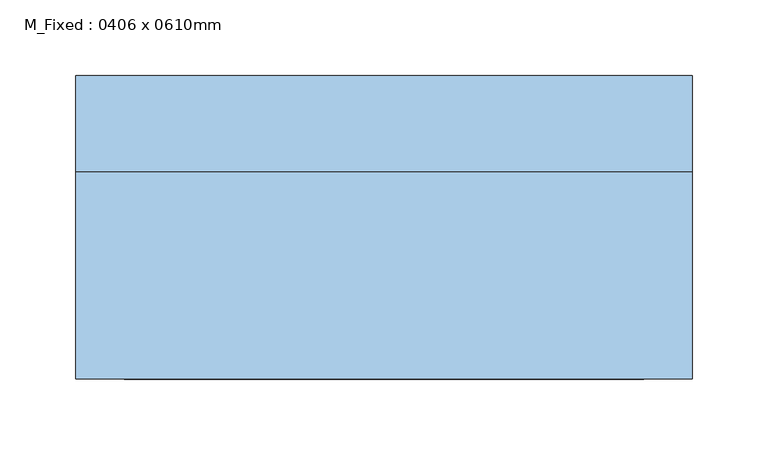
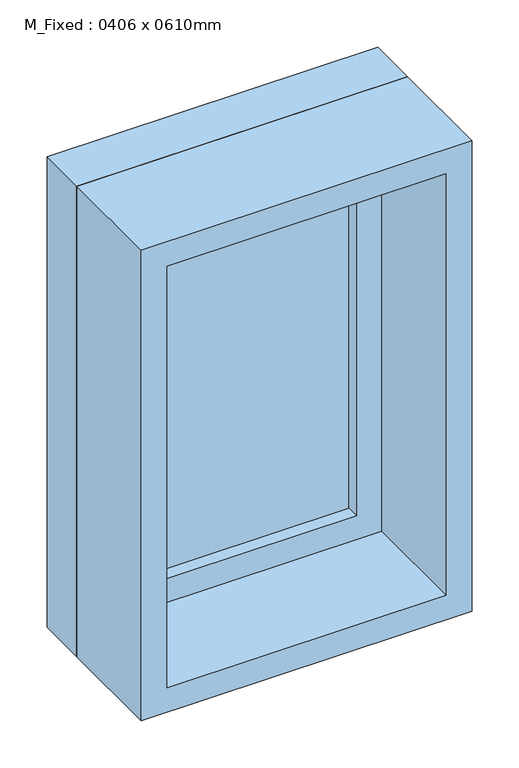
"""IFC4 building model written with IfcOpenShell, lengths in millimetres: window geometry, M_Fixed : 0406 x 0610mm."""

from ifc_helpers import new_model, si_unit, frame, origin, place, context, project, spatial, polyline, outline, extrude, source, transform, mapped, element, save


def m_fixed_0406_x_0610mm_8205b201(model_context):
    return source(origin(), model_context, "Body", "SweptSolid", [
        extrude(outline(polyline([(-140.0, 78.0), (140.0, 78.0), (140.0, 66.0), (-140.0, 66.0), (-140.0, 78.0)])), frame((0.0, 0.0, 978.0), z_axis=(0.0, 0.0, 1.0), x_axis=(1.0, 0.0, 0.0)), (0.0, 0.0, 1.0), 484.0),
        extrude(outline(polyline([(1506.0, -184.0), (934.0, -184.0), (934.0, 184.0), (1506.0, 184.0), (1506.0, -184.0)]), holes=[polyline([(1462.0, -140.0), (1462.0, 140.0), (978.0, 140.0), (978.0, -140.0), (1462.0, -140.0)])]), frame((0.0, 50.0, 0.0), z_axis=(0.0, 1.0, 0.0), x_axis=(0.0, 0.0, 1.0)), (0.0, 0.0, 1.0), 44.0),
        extrude(outline(polyline([(1525.0, -203.0), (915.0, -203.0), (915.0, 203.0), (1525.0, 203.0), (1525.0, -203.0)]), holes=[polyline([(1506.0, -184.0), (1506.0, 184.0), (934.0, 184.0), (934.0, -184.0), (1506.0, -184.0)])]), frame((0.0, 50.0, 0.0), z_axis=(0.0, 1.0, 0.0), x_axis=(0.0, 0.0, 1.0)), (0.0, 0.0, 1.0), 63.0),
        extrude(outline(polyline([(1525.0, -203.0), (915.0, -203.0), (915.0, 203.0), (1525.0, 203.0), (1525.0, -203.0)]), holes=[polyline([(1493.0, -171.0), (1493.0, 171.0), (947.0, 171.0), (947.0, -171.0), (1493.0, -171.0)])]), frame((0.0, -87.0, 0.0), z_axis=(0.0, 1.0, 0.0), x_axis=(0.0, 0.0, 1.0)), (0.0, 0.0, 1.0), 137.0),
    ])


if __name__ == "__main__":
    model = new_model("IFC4")
    model_context = context("Model", 3, world=origin())
    ifc_project = project(units=[si_unit("LENGTHUNIT", "METRE", prefix="MILLI")], contexts=[model_context])
    site = spatial("IfcSite", under=ifc_project)
    building = spatial("IfcBuilding", under=site)
    placement = place(None, origin())
    m_fixed_0406_x_0610mm_shape = m_fixed_0406_x_0610mm_8205b201(model_context)
    element("IfcWindow", 1, ObjectType="M_Fixed : 0406 x 0610mm", at=placement, inside=building, context=model_context, shape_type="MappedRepresentation", body=[
        mapped(m_fixed_0406_x_0610mm_shape, transform((0.0, 0.0, 0.0), x_axis=(1.0, 0.0, 0.0), y_axis=(0.0, 1.0, 0.0), z_axis=(0.0, 0.0, 1.0))),
    ])
    save(model, "model.ifc")

# Revit data of these elements
# Type "M_Fixed : 0406 x 0610mm"
#   Type Mark = "10"
#   Height = 610 mm
#   Default Sill Height = 915 mm
#   Width = 406 mm
#   Window Inset = 19 mm
#   Frame Exterior Material = Sash
#   Frame Interior Material = Sash
#   Glass Pane Material = Glass
#   Sash = Sash
#   Wall Closure = (empty or 0)
# Element 1 (IfcWindow, "M_Fixed : 0406 x 0610mm")
#   Materials on its faces: "Sash", "Glass"
# Materials
#   "Sash": class "Wood", colour RGB 136 99 55, transparency 0
#   "Glass": class "Glass", colour RGB 218 227 224, transparency 0.85, Description = "Soda Lime Glass", Cost = 0
